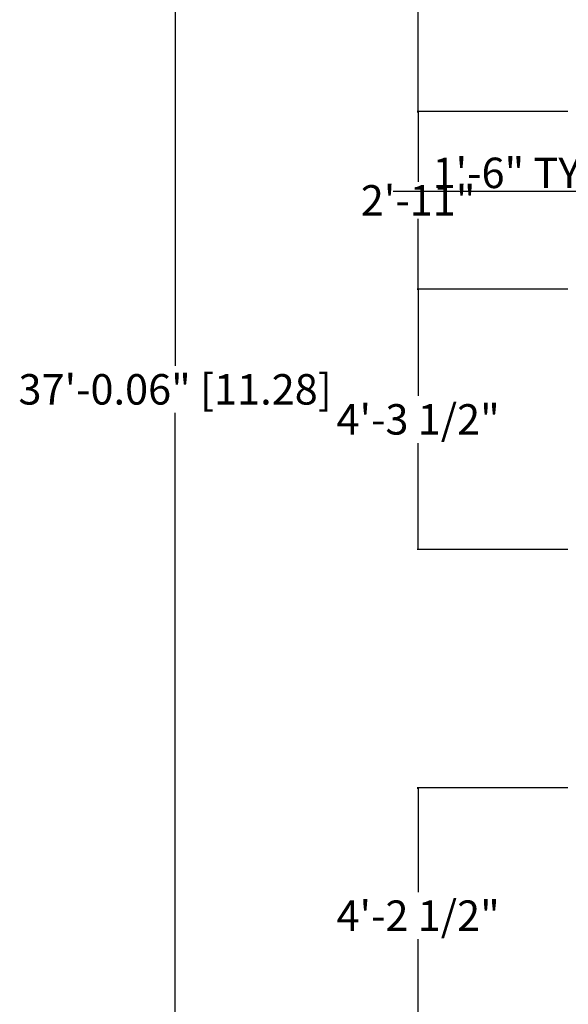
# Model space of a CAD drawing. Units: inches. Extents: x 2322 to 2932, y 142 to 762.
# Tile 3 of 7: x 2322 to 2430, y 376 to 570. Entities that reach past the tile are written whole.
import ezdxf

# ---------------------------------------------------------------- set-up
doc = ezdxf.new("R2010")
doc.units = ezdxf.units.IN
doc.header["$MEASUREMENT"] = 0
doc.layers.add('A-ANNO-DIMS', color=2, linetype='Continuous', lineweight=18)
doc.styles.get("Standard").update_dxf_attribs({"font": 'italic8.shx'})
doc.dimstyles.get("Standard").update_dxf_attribs({"dimtxt": 6, "dimasz": 0.15, "dimexe": 0.18, "dimexo": 0.0625, "dimgap": 0.09, "dimtad": 1, "dimtih": 1, "dimtoh": 1, "dimzin": 0, "dimdsep": 46, "dimlunit": 3, "dimtxsty": 'Standard', "dimblk": 'CLOSEDBLANK', "dimcen": 0.09, "dimclrd": 3, "dimclre": 1, "dimclrt": 6, "dimadec": 0, "dimazin": 0, "dimtfac": 1, "dimtofl": 0, "dimtmove": 0, "dimatfit": 3, "dimldrblk": 'DOT', "dimfxl": 1, "dimtolj": 1, "dimtzin": 0, "dimarcsym": 0})

# ---------------------------------------------------------------- blocks, each defined once
blk = doc.blocks.new('_ClosedBlank')
at = {"color": 0, "linetype": 'ByBlock', "lineweight": -2}
for p, q in [((-1, 0.2), (0, 0)), ((-1, 0.2), (-1, -0.2)), ((0, 0), (-1, -0.2))]:
    blk.add_line(p, q, dxfattribs=at)
blk = doc.blocks.new('*D8')
at = {"layer": 'A-ANNO-DIMS', "color": 0, "lineweight": -2, "transparency": 16777216}
for p, q in [((2430, 718.82), (2352.33, 718.82)), ((2352.51, 718.67), (2352.51, 501.45)), ((2352.51, 274.91), (2352.51, 492.13)), ((2430, 274.76), (2352.33, 274.76))]:
    blk.add_line(p, q, dxfattribs=at)
at = {"layer": 'Defpoints', "color": 0, "transparency": 16777216}
for p in [(2430.06, 718.82), (2352.51, 274.76), (2430.06, 274.76)]:
    blk.add_point(p, dxfattribs=at)
at = {"layer": 'A-ANNO-DIMS', "color": 0, "lineweight": -2, "transparency": 16777216, "xscale": 0.15, "yscale": 0.15, "zscale": 0.15}
for p, rotation in [((2352.51, 718.82), 90), ((2352.51, 274.76), 270)]:
    blk.add_blockref('_ClosedBlank', p, dxfattribs=dict(at, rotation=rotation))
at = {"layer": 'A-ANNO-DIMS', "color": 0, "transparency": 16777216, "insert": (2352.51, 496.79), "char_height": 6, "attachment_point": 5}
blk.add_mtext('\\A1;37\'-0.06" [11.28]', dxfattribs=at)
blk = doc.blocks.new('_Dot')
at = {"color": 0, "linetype": 'ByBlock', "lineweight": -2}
blk.add_line((-0.5, 0), (-1, 0), dxfattribs=at)
at = {"color": 0, "linetype": 'ByBlock', "const_width": 0.5}
blk.add_lwpolyline([(-0.25, 0, 1), (0.25, 0, 1)], format="xyb", close=True, dxfattribs=at)
blk = doc.blocks.new('*D37')
at = {"layer": 'A-ANNO-DIMS', "color": 1, "lineweight": -2, "transparency": 16777216}
for p, q in [((2447.84, 531.38), (2447.84, 536)), ((2465.84, 531.38), (2465.84, 536))]:
    blk.add_line(p, q, dxfattribs=at)
at = {"layer": 'A-ANNO-DIMS', "color": 3, "lineweight": -2, "transparency": 16777216}
for p, q in [((2447.84, 535.82), (2395.51, 535.82)), ((2465.69, 535.82), (2447.99, 535.82))]:
    blk.add_line(p, q, dxfattribs=at)
at = {"layer": 'Defpoints', "color": 0, "transparency": 16777216}
for p in [(2447.84, 535.82), (2447.84, 531.32), (2465.84, 531.32)]:
    blk.add_point(p, dxfattribs=at)
at = {"layer": 'A-ANNO-DIMS', "color": 3, "lineweight": -2, "transparency": 16777216, "xscale": 0.15, "yscale": 0.15, "zscale": 0.15, "rotation": 180}
blk.add_blockref('_ClosedBlank', (2447.84, 535.82), dxfattribs=at)
at = {"layer": 'A-ANNO-DIMS', "color": 3, "lineweight": -2, "transparency": 16777216, "xscale": 0.15, "yscale": 0.15, "zscale": 0.15}
blk.add_blockref('_ClosedBlank', (2465.84, 535.82), dxfattribs=at)
at = {"layer": 'A-ANNO-DIMS', "color": 6, "transparency": 16777216, "insert": (2421.6, 539.48), "char_height": 6, "attachment_point": 5}
blk.add_mtext('\\A1;1\'-6" TYP.', dxfattribs=at)
blk = doc.blocks.new('*D57')
at = {"layer": 'A-ANNO-DIMS', "color": 1, "lineweight": -2, "transparency": 16777216}
for p, q in [((2430, 418.18), (2400.26, 418.18)), ((2439, 367.82), (2400.26, 367.82))]:
    blk.add_line(p, q, dxfattribs=at)
at = {"layer": 'A-ANNO-DIMS', "color": 3, "lineweight": -2, "transparency": 16777216}
for p, q in [((2400.44, 418.03), (2400.44, 397.66)), ((2400.44, 367.97), (2400.44, 388.34))]:
    blk.add_line(p, q, dxfattribs=at)
at = {"layer": 'Defpoints', "color": 0, "transparency": 16777216}
for p in [(2400.44, 418.18), (2430.06, 418.18), (2439.06, 367.82)]:
    blk.add_point(p, dxfattribs=at)
at = {"layer": 'A-ANNO-DIMS', "color": 3, "lineweight": -2, "transparency": 16777216, "xscale": 0.15, "yscale": 0.15, "zscale": 0.15}
for p, rotation in [((2400.44, 418.18), 90), ((2400.44, 367.82), 270)]:
    blk.add_blockref('_ClosedBlank', p, dxfattribs=dict(at, rotation=rotation))
at = {"layer": 'A-ANNO-DIMS', "color": 6, "transparency": 16777216, "insert": (2400.44, 393), "char_height": 6, "attachment_point": 5}
blk.add_mtext('\\A1;4\'-2 1/2"', dxfattribs=at)
blk = doc.blocks.new('*D58')
at = {"layer": 'A-ANNO-DIMS', "color": 1, "lineweight": -2, "transparency": 16777216}
for p, q in [((2430, 516.56), (2400.26, 516.56)), ((2430, 465.18), (2400.26, 465.18))]:
    blk.add_line(p, q, dxfattribs=at)
at = {"layer": 'A-ANNO-DIMS', "color": 3, "lineweight": -2, "transparency": 16777216}
for p, q in [((2400.44, 516.41), (2400.44, 495.53)), ((2400.44, 465.33), (2400.44, 486.21))]:
    blk.add_line(p, q, dxfattribs=at)
at = {"layer": 'Defpoints', "color": 0, "transparency": 16777216}
for p in [(2400.44, 516.56), (2430.06, 516.56), (2430.06, 465.18)]:
    blk.add_point(p, dxfattribs=at)
at = {"layer": 'A-ANNO-DIMS', "color": 3, "lineweight": -2, "transparency": 16777216, "xscale": 0.15, "yscale": 0.15, "zscale": 0.15}
for p, rotation in [((2400.44, 516.56), 90), ((2400.44, 465.18), 270)]:
    blk.add_blockref('_ClosedBlank', p, dxfattribs=dict(at, rotation=rotation))
at = {"layer": 'A-ANNO-DIMS', "color": 6, "transparency": 16777216, "insert": (2400.44, 490.87), "char_height": 6, "attachment_point": 5}
blk.add_mtext('\\A1;4\'-3 1/2"', dxfattribs=at)
blk = doc.blocks.new('*D59')
at = {"layer": 'A-ANNO-DIMS', "color": 1, "lineweight": -2, "transparency": 16777216}
for p, q in [((2430, 551.56), (2400.26, 551.56)), ((2430, 516.56), (2400.26, 516.56))]:
    blk.add_line(p, q, dxfattribs=at)
at = {"layer": 'A-ANNO-DIMS', "color": 3, "lineweight": -2, "transparency": 16777216}
for p, q in [((2400.44, 551.41), (2400.44, 537.72)), ((2400.44, 516.71), (2400.44, 530.4))]:
    blk.add_line(p, q, dxfattribs=at)
at = {"layer": 'Defpoints', "color": 0, "transparency": 16777216}
for p in [(2400.44, 551.56), (2430.06, 551.56), (2430.06, 516.56)]:
    blk.add_point(p, dxfattribs=at)
at = {"layer": 'A-ANNO-DIMS', "color": 3, "lineweight": -2, "transparency": 16777216, "xscale": 0.15, "yscale": 0.15, "zscale": 0.15}
for p, rotation in [((2400.44, 551.56), 90), ((2400.44, 516.56), 270)]:
    blk.add_blockref('_ClosedBlank', p, dxfattribs=dict(at, rotation=rotation))
at = {"layer": 'A-ANNO-DIMS', "color": 6, "transparency": 16777216, "insert": (2400.44, 534.06), "char_height": 6, "attachment_point": 5}
blk.add_mtext('\\A1;2\'-11"', dxfattribs=at)
blk = doc.blocks.new('*D60')
at = {"layer": 'A-ANNO-DIMS', "color": 1, "lineweight": -2, "transparency": 16777216}
for p, q in [((2430, 616.55), (2400.26, 616.55)), ((2430, 551.56), (2400.26, 551.56))]:
    blk.add_line(p, q, dxfattribs=at)
at = {"layer": 'A-ANNO-DIMS', "color": 3, "lineweight": -2, "transparency": 16777216}
for p, q in [((2400.44, 616.4), (2400.44, 587.72)), ((2400.44, 551.71), (2400.44, 580.39))]:
    blk.add_line(p, q, dxfattribs=at)
at = {"layer": 'Defpoints', "color": 0, "transparency": 16777216}
for p in [(2400.44, 616.55), (2430.06, 616.55), (2430.06, 551.56)]:
    blk.add_point(p, dxfattribs=at)
at = {"layer": 'A-ANNO-DIMS', "color": 3, "lineweight": -2, "transparency": 16777216, "xscale": 0.15, "yscale": 0.15, "zscale": 0.15}
for p, rotation in [((2400.44, 616.55), 90), ((2400.44, 551.56), 270)]:
    blk.add_blockref('_ClosedBlank', p, dxfattribs=dict(at, rotation=rotation))
at = {"layer": 'A-ANNO-DIMS', "color": 6, "transparency": 16777216, "insert": (2400.44, 584.06), "char_height": 6, "attachment_point": 5}
blk.add_mtext('\\A1;5\'-5"', dxfattribs=at)

msp = doc.modelspace()

# ---------------------------------------------------------------- dimensions: what is measured, and where the dimension line sits
at = {"layer": 'A-ANNO-DIMS'}
for base, p1, p2, override, picture, middle in [((2352.512, 274.756), (2430.065, 718.819), (2430.065, 274.756), {"dimclrd": 0, "dimclre": 0, "dimclrt": 0}, '*D8', (2352.512, 496.787)), ((2400.44, 616.548), (2430.065, 551.562), (2430.065, 616.548), {"dimdec": 1, "dimlfac": 1, "dimrnd": 0, "dimzin": 1, "dimdsep": 46, "dimlunit": 4, "dimfrac": 2}, '*D60', (2400.44, 584.055)), ((2400.44, 551.562), (2430.065, 516.562), (2430.065, 551.562), {"dimdec": 1, "dimlfac": 1, "dimrnd": 0, "dimzin": 1, "dimdsep": 46, "dimlunit": 4, "dimfrac": 2}, '*D59', (2400.44, 534.062)), ((2400.44, 516.562), (2430.065, 465.181), (2430.065, 516.562), {"dimdec": 1, "dimlfac": 1, "dimrnd": 0, "dimzin": 1, "dimdsep": 46, "dimlunit": 4, "dimfrac": 2}, '*D58', (2400.44, 490.872)), ((2400.44, 418.181), (2439.065, 367.819), (2430.065, 418.181), {"dimdec": 1, "dimlfac": 1, "dimrnd": 0, "dimzin": 1, "dimdsep": 46, "dimlunit": 4, "dimfrac": 2}, '*D57', (2400.44, 393))]:
    dim = msp.add_linear_dim(base=base, p1=p1, p2=p2, angle=90, dimstyle='Standard', override=override, dxfattribs=at)
    dim.commit()
    dim.dimension.update_dxf_attribs({"geometry": picture, "text_midpoint": middle})
dim = msp.add_linear_dim(base=(2447.837, 535.819), p1=(2465.837, 531.319), p2=(2447.837, 531.319), angle=180, text='<> TYP.', dimstyle='Standard', override={"dimdec": 1, "dimlfac": 1, "dimrnd": 0, "dimzin": 1, "dimdsep": 46, "dimlunit": 4, "dimfrac": 2}, dxfattribs=at)
dim.commit()
dim.dimension.update_dxf_attribs({"geometry": '*D37', "text_midpoint": (2421.597, 539.48)})

doc.saveas('drawing.dxf')
